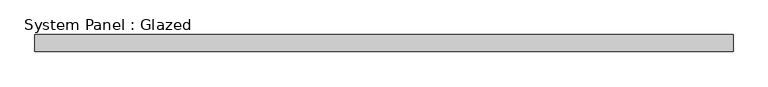
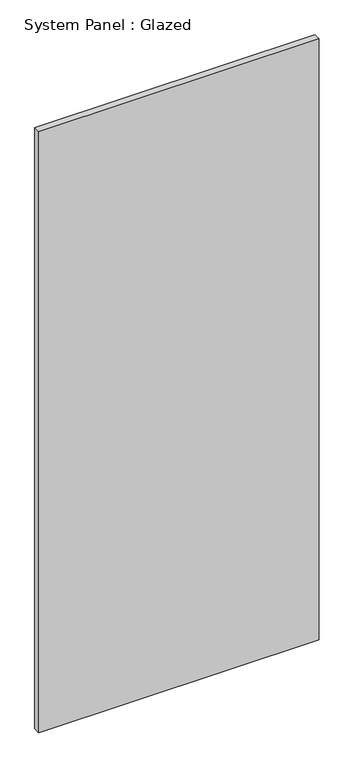
"""IFC4 building model written with IfcOpenShell, lengths in millimetres: plate geometry, System Panel : Glazed."""

from ifc_helpers import new_model, si_unit, origin, origin_with_axes, place, context, project, spatial, polyline, outline, extrude, source, transform, mapped, element, save


def system_panel_glazed_66ef8e2c(model_context):
    return source(origin(), model_context, "Body", "SweptSolid", [
        extrude(outline(polyline([(523.875, 19.05), (-523.875, 19.05), (-523.875, 44.45), (523.875, 44.45), (523.875, 19.05)])), origin_with_axes(), (0.0, 0.0, 1.0), 2374.9),
    ])


if __name__ == "__main__":
    model = new_model("IFC4")
    model_context = context("Model", 3, world=origin())
    ifc_project = project(units=[si_unit("LENGTHUNIT", "METRE", prefix="MILLI")], contexts=[model_context])
    site = spatial("IfcSite", under=ifc_project)
    building = spatial("IfcBuilding", under=site)
    placement = place(None, origin())
    system_panel_glazed_shape = system_panel_glazed_66ef8e2c(model_context)
    element("IfcPlate", 1, ObjectType="System Panel : Glazed", at=placement, inside=building, context=model_context, shape_type="MappedRepresentation", body=[
        mapped(system_panel_glazed_shape, transform((0.0, 0.0, 0.0), x_axis=(1.0, 0.0, 0.0), y_axis=(0.0, 1.0, 0.0), z_axis=(0.0, 0.0, 1.0))),
    ])
    save(model, "model.ifc")

# Revit data of these elements
# Type "System Panel : Glazed"
#   Construction Type Id = "GSP4R"
#   Analytic Construction = "1/8 in Pilkington single glazing"
#   Visual Light Transmittance = 0.9
#   Solar Heat Gain Coefficient = 0.86
#   Heat Transfer Coefficient (U) = 1.18115 BTU/(h·ft²·°F)
# Element 1 (IfcPlate, "System Panel : Glazed")
#   Materials on its faces: "Glass"
# Materials
#   "Glass": class "Glass", colour RGB 0 128 192, transparency 0.75, Description = "Soda Lime Glass", Cost = 0
